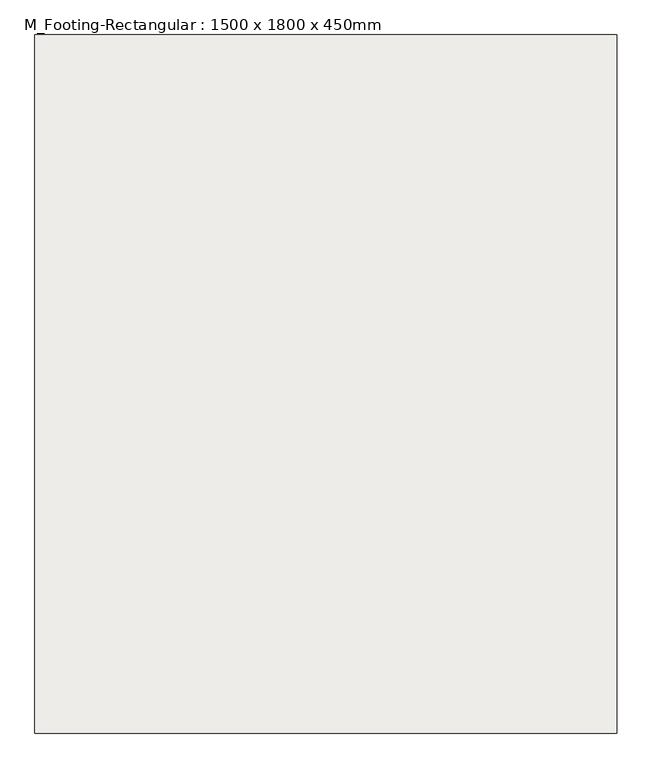
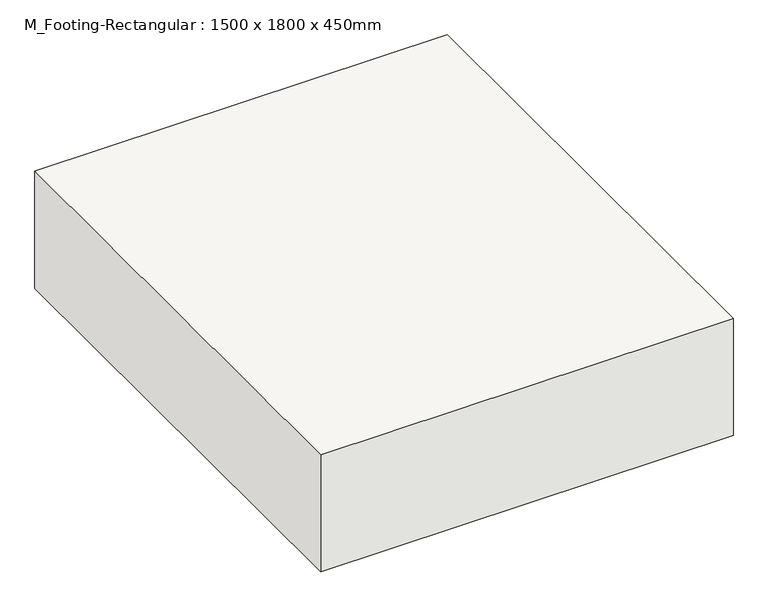
"""IFC4 building model written with IfcOpenShell, lengths in millimetres: slab geometry, M_Footing-Rectangular : 1500 x 1800 x 450mm."""

from ifc_helpers import new_model, si_unit, frame, origin, place, context, project, spatial, polyline, outline, extrude, source, transform, mapped, element, save


def m_footing_rectangular_1500_x_1800_x_450mm_b88d8e73(model_context):
    return source(origin(), model_context, "Body", "SweptSolid", [
        extrude(outline(polyline([(750.0, 900.0), (750.0, -900.0), (-750.0, -900.0), (-750.0, 900.0), (750.0, 900.0)])), frame((0.0, 0.0, -450.0), z_axis=(0.0, 0.0, 1.0), x_axis=(1.0, 0.0, 0.0)), (0.0, 0.0, 1.0), 450.0),
    ])


if __name__ == "__main__":
    model = new_model("IFC4")
    model_context = context("Model", 3, world=origin())
    ifc_project = project(units=[si_unit("LENGTHUNIT", "METRE", prefix="MILLI")], contexts=[model_context])
    site = spatial("IfcSite", under=ifc_project)
    building = spatial("IfcBuilding", under=site)
    placement = place(None, origin())
    m_footing_rectangular_1500_x_1800_x_450mm_shape = m_footing_rectangular_1500_x_1800_x_450mm_b88d8e73(model_context)
    element("IfcSlab", 1, ObjectType="M_Footing-Rectangular : 1500 x 1800 x 450mm", at=placement, inside=building, context=model_context, shape_type="MappedRepresentation", body=[
        mapped(m_footing_rectangular_1500_x_1800_x_450mm_shape, transform((0.0, 0.0, 0.0), x_axis=(1.0, 0.0, 0.0), y_axis=(0.0, 1.0, 0.0), z_axis=(0.0, 0.0, 1.0))),
    ])
    save(model, "model.ifc")

# Revit data of these elements
# Type "M_Footing-Rectangular : 1500 x 1800 x 450mm"
#   Width = 4' - 11.05512"
#   Length = 5' - 10.86614"
#   Foundation Thickness = 1' - 5.71654"
#   Structural Material [instance default] = Concrete, Cast-in-Place gray
#   Assembly Code = ""
# Element 1 (IfcSlab, "M_Footing-Rectangular : 1500 x 1800 x 450mm")
#   Materials on its faces: "Concrete, Cast-in-Place gray"
# Materials
#   "Concrete, Cast-in-Place gray": class "Concrete", colour RGB 192 192 192, transparency 0, Description = "Cast-in-place concrete", Cost = 0
